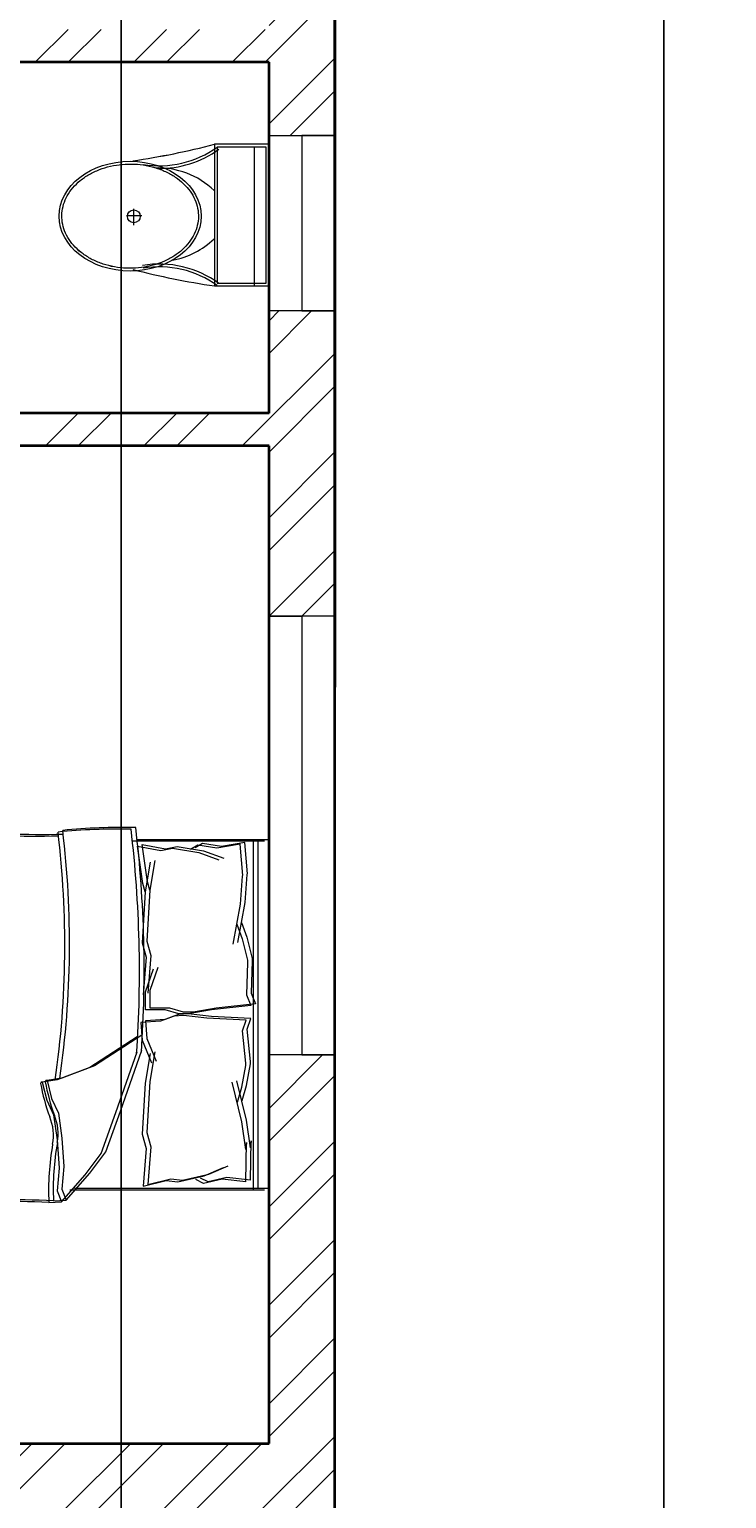
# Model space of a CAD drawing. Units: inches. Extents: x 2120 to 4013, y 1390 to 3019.
# Tile 43 of 59: x 2968 to 3063, y 1964 to 2165. Entities that reach past the tile are written whole.
import ezdxf

# ---------------------------------------------------------------- set-up
doc = ezdxf.new("R2010")
doc.units = ezdxf.units.IN
for name, color, linetype, lineweight in [('A-ANNO-DIMS', 2, 'Continuous', 18), ('A-FLOR-FIXT', 9, 'Continuous', 18), ('A-FURN', 8, 'Continuous', 13), ('A-GLAZ', 4, 'Continuous', 18), ('A-WALL', 7, 'Continuous', 35), ('A-WALL-PATT', 252, 'Continuous', 13)]:
    doc.layers.add(name, color=color, linetype=linetype, lineweight=lineweight)
doc.styles.get("Standard").update_dxf_attribs({"font": 'arial.ttf'})
doc.dimstyles.get("Standard").update_dxf_attribs({"dimtxt": 0.18, "dimasz": 0.18, "dimexe": 0.18, "dimexo": 0.0625, "dimgap": 0.09, "dimtad": 0, "dimtih": 1, "dimtoh": 1, "dimdec": 4, "dimzin": 0, "dimdsep": 46, "dimtxsty": 'Standard', "dimcen": 0.09, "dimadec": 0, "dimazin": 0, "dimtfac": 1, "dimtdec": 4, "dimtofl": 0, "dimtmove": 0, "dimatfit": 3, "dimfxl": 1, "dimtolj": 1, "dimtzin": 0, "dimarcsym": 0})

# ---------------------------------------------------------------- blocks, each defined once
blk = doc.blocks.new('A$C31115884')
for p, q in [((283.1, 497.7), (223.4, 497.7)), ((257.5, 466.4), (257.5, 523.2)), ((0, 200), (0, 0)), ((520, 200), (0, 200)), ((10, 190), (10, 10)), ((510, 190), (10, 190)), ((510, 10), (510, 190)), ((520, 0), (520, 200)), ((510, 54.5), (0, 54.5)), ((10, 10), (510, 10)), ((0, 0), (520, 0))]:
    blk.add_line(p, q)
blk.add_circle((255.6, 496.4), 23.6)
for centre, radius, start, end in [((2777.7, -204.6), 2807, 165.4549, 171.7133), ((3237, 905), 2807, 188.2867, 194.5451), ((-294.5, 403.3), 364.7, 324.2091, 9.3499), ((-294.5, 403.3), 374.7, 324.2091, 9.3499), ((805.8, 403.3), 364.7, 170.6501, 215.7909), ((139.5, 406.2), 293.5, 315.8436, 2.6563), ((805.8, 403.3), 374.7, 179.2036, 215.7909), ((383.6, 406.2), 293.5, 190.2774, 224.1564)]:
    blk.add_arc(centre, radius, start, end)
blk.add_ellipse((256.2, 509.9), major_axis=(0, -260.7), ratio=0.772727)
blk.add_open_spline([(256.2, 259.2), (263.1, 259.2), (270, 259.7), (287.8, 262.3), (298.7, 265.1), (319.9, 273.1), (330.2, 278.4), (350.1, 291.1), (359.7, 298.7), (377.7, 315.9), (386.2, 325.5), (401.7, 346.6), (408.8, 358.1), (421.3, 382.5), (426.8, 395.5), (435.9, 422.4), (439.5, 436.4), (444.8, 465.1), (446.5, 479.7), (447.9, 509.2), (447.6, 524), (445, 553.3), (442.7, 567.8), (436.3, 596), (432.1, 609.7), (421.9, 636), (416, 648.6), (402.5, 672.1), (395, 683), (378.6, 703), (369.8, 712.1), (351.1, 728), (341.3, 734.8), (320.9, 746.2), (310.4, 750.7), (288.9, 757.3), (278, 759.4), (256, 761), (245, 760.6), (223.1, 757.2), (212.3, 754.3), (191.1, 746.1), (180.8, 740.7), (160.9, 727.8), (151.4, 720.1), (133.5, 702.7), (125.1, 693), (109.6, 671.7), (102.6, 660.2), (90.2, 635.7), (84.9, 622.7), (76, 595.6), (72.4, 581.6), (67.2, 552.9), (65.6, 538.2), (64.4, 508.8), (64.8, 494), (67.5, 464.7), (69.9, 450.2), (76.6, 422), (80.8, 408.3), (91.1, 382.2), (97.2, 369.7), (110.8, 346.3), (118.4, 335.4), (134.8, 315.6), (143.7, 306.7), (162.4, 290.9), (172.3, 284.2), (192.8, 273), (203.3, 268.6), (224.8, 262.2), (235.8, 260.2), (249.9, 259.3), (253, 259.2), (256.2, 259.2)], degree=3, knots=[0, 0, 0, 0, 0.110105, 0.110105, 0.285049, 0.285049, 0.459994, 0.459994, 0.634938, 0.634938, 0.809882, 0.809882, 0.984827, 0.984827, 1.159771, 1.159771, 1.334715, 1.334715, 1.50966, 1.50966, 1.684604, 1.684604, 1.859549, 1.859549, 2.034493, 2.034493, 2.209437, 2.209437, 2.384382, 2.384382, 2.559326, 2.559326, 2.73427, 2.73427, 2.909215, 2.909215, 3.084159, 3.084159, 3.259103, 3.259103, 3.434048, 3.434048, 3.608992, 3.608992, 3.783936, 3.783936, 3.958881, 3.958881, 4.133825, 4.133825, 4.30877, 4.30877, 4.483714, 4.483714, 4.658658, 4.658658, 4.833603, 4.833603, 5.008547, 5.008547, 5.183491, 5.183491, 5.358436, 5.358436, 5.53338, 5.53338, 5.708324, 5.708324, 5.883269, 5.883269, 6.058213, 6.058213, 6.233158, 6.233158, 6.283185, 6.283185, 6.283185, 6.283185])
blk = doc.blocks.new('BED-DOUBLE-PLAN')
for p, q in [((3.48, 63.34), (3.48, 81.45)), ((3.48, 81.45), (51.27, 81.45)), ((3.7, 62.7), (3.7, 80.81)), ((51.27, 81.45), (51.27, 54.84)), ((51.5, 80.81), (51.5, 54.2)), ((3.48, 79.91), (51.27, 79.91)), ((3.7, 79.27), (51.5, 79.27)), ((3.9, 78.11), (8.18, 78.44)), ((8.18, 78.44), (8.29, 78.42)), ((8.29, 78.42), (12.11, 78.13)), ((14.86, 77.7), (16.88, 78.42)), ((16.88, 78.42), (19.77, 79.14)), ((17.11, 77.78), (20, 78.5)), ((19.77, 79.14), (20.09, 79.14)), ((20, 78.5), (20.32, 78.5)), ((20.09, 79.14), (24.54, 79)), ((20.32, 78.5), (24.77, 78.36)), ((24.54, 79), (25.98, 79.58)), ((24.77, 78.36), (26.21, 78.94)), ((25.98, 79.58), (26.56, 74.23)), ((26.21, 78.94), (26.79, 73.59)), ((27.98, 78.95), (27.73, 73.58)), ((29.46, 78.47), (27.98, 78.95)), ((33.89, 78.89), (29.46, 78.47)), ((34.21, 78.91), (33.89, 78.89)), ((37.14, 78.37), (34.21, 78.91)), ((45.71, 78.9), (41.92, 78.38)), ((50.11, 78.89), (44.71, 78.99)), ((44.71, 78.99), (45.71, 78.9)), ((50.11, 78.89), (49.73, 75.68)), ((3.9, 78.13), (4.47, 74.95)), ((4.12, 77.49), (4.7, 74.31)), ((4.13, 77.47), (8.41, 77.8)), ((8.41, 77.8), (8.51, 77.78)), ((8.51, 77.78), (12.34, 77.49)), ((12.11, 78.13), (17.6, 77.12)), ((12.34, 77.49), (17.83, 76.48)), ((15.08, 77.06), (17.11, 77.78)), ((28.21, 78.32), (27.96, 72.94)), ((29.69, 77.83), (28.21, 78.32)), ((34.11, 78.25), (29.69, 77.83)), ((34.43, 78.27), (34.11, 78.25)), ((37.37, 77.73), (34.43, 78.27)), ((41.92, 78.38), (36.5, 77.02)), ((42.14, 77.74), (36.72, 76.38)), ((39.2, 77.77), (37.14, 78.37)), ((39.43, 77.13), (37.37, 77.73)), ((45.94, 78.26), (42.14, 77.74)), ((50.34, 78.25), (44.94, 78.35)), ((44.94, 78.35), (45.94, 78.26)), ((50.34, 78.25), (49.96, 75.04)), ((4.47, 74.95), (4.04, 72.35)), ((5.05, 72.49), (6.06, 75.24)), ((5.28, 71.85), (6.29, 74.6)), ((49.31, 73.19), (48.13, 75.87)), ((49.54, 72.55), (48.36, 75.23)), ((49.73, 75.68), (50.33, 73.11)), ((49.96, 75.04), (50.56, 72.47)), ((4.7, 74.31), (4.27, 71.71)), ((4.47, 68.88), (5.05, 72.49)), ((26.56, 74.23), (27.14, 71.05)), ((26.79, 73.59), (27.37, 70.41)), ((27.73, 73.58), (27.36, 70.37)), ((27.96, 72.94), (27.58, 69.73)), ((50.11, 69.62), (49.31, 73.19)), ((50.34, 68.98), (49.54, 72.55)), ((50.33, 73.11), (49.82, 72.06)), ((50.56, 72.47), (50.04, 71.42)), ((4.04, 72.35), (4.62, 71.33)), ((4.27, 71.71), (4.85, 70.7)), ((4.7, 68.24), (5.28, 71.85)), ((27.14, 71.05), (27.14, 69.74)), ((27.36, 70.37), (27.44, 69.07)), ((27.37, 70.41), (27.37, 69.1)), ((4.76, 67.29), (4.47, 68.88)), ((27.14, 69.74), (26.56, 67.86)), ((27.37, 69.1), (26.79, 67.23)), ((27.44, 69.07), (28.13, 67.23)), ((27.58, 69.73), (27.67, 68.43)), ((27.67, 68.43), (28.36, 66.59)), ((49.92, 68.01), (50.11, 69.62)), ((50.15, 67.37), (50.34, 68.98)), ((4.19, 64.11), (4.76, 67.29)), ((4.41, 63.47), (4.99, 66.65)), ((4.99, 66.65), (4.7, 68.24)), ((26.56, 67.86), (26.56, 65.18)), ((26.79, 67.23), (26.79, 64.54)), ((28.13, 67.23), (28.3, 64.55)), ((28.36, 66.59), (28.53, 63.91)), ((50.7, 64.87), (49.92, 68.01)), ((50.93, 64.23), (50.15, 67.37)), ((9.28, 64.83), (4.19, 64.11)), ((6.38, 65.82), (10.42, 65.15)), ((6.61, 65.18), (10.64, 64.51)), ((10.42, 65.15), (9.28, 64.83)), ((10.64, 64.51), (9.51, 64.19)), ((10.42, 65.15), (17.43, 64.72)), ((10.64, 64.51), (17.65, 64.08)), ((17.43, 64.72), (19.39, 65.28)), ((17.65, 64.08), (19.61, 64.64)), ((19.39, 65.28), (24.52, 64.87)), ((19.61, 64.64), (24.75, 64.23)), ((24.1, 65.18), (20.96, 66.27)), ((24.33, 64.54), (21.19, 65.63)), ((26.56, 65.18), (24.1, 65.18)), ((26.79, 64.54), (24.33, 64.54)), ((28.3, 64.55), (30.75, 64.71)), ((30.75, 64.71), (33.82, 65.99)), ((30.98, 64.07), (34.05, 65.35)), ((32.57, 65.82), (36.6, 65.15)), ((32.79, 65.18), (36.83, 64.51)), ((36.6, 65.15), (43.61, 64.72)), ((36.83, 64.51), (43.84, 64.08)), ((43.61, 64.72), (45.57, 65.28)), ((43.84, 64.08), (45.8, 64.64)), ((45.57, 65.28), (50.7, 64.87)), ((45.8, 64.64), (50.93, 64.23)), ((9.51, 64.19), (4.41, 63.47)), ((28.53, 63.91), (30.98, 64.07)), ((30.26, 64.06), (34.45, 57.57)), ((30.49, 63.42), (34.68, 56.93)), ((40.65, 61.13), (32.31, 64.06)), ((40.87, 60.49), (32.54, 63.42)), ((46.22, 59.12), (40.65, 61.13)), ((46.45, 58.48), (40.87, 60.49)), ((49.16, 56.95), (46.22, 59.12)), ((49.39, 56.31), (46.45, 58.48)), ((34.45, 57.57), (36.15, 53.08)), ((34.68, 56.93), (36.38, 52.44)), ((52.87, 53.7), (49.16, 56.95)), ((53.1, 53.06), (49.39, 56.31)), ((36.15, 53.08), (36.46, 51.07)), ((36.38, 52.44), (36.69, 50.43)), ((38.94, 51.69), (40.96, 52.62)), ((40.96, 52.62), (44.36, 53.08)), ((41.18, 51.98), (44.59, 52.44)), ((44.36, 53.08), (48.23, 53.39)), ((44.59, 52.44), (48.46, 52.75)), ((48.23, 53.39), (51.33, 53.08)), ((48.46, 52.75), (51.56, 52.44)), ((51.33, 53.08), (52.87, 53.7)), ((51.56, 52.44), (53.1, 53.06)), ((52.95, 51.96), (52.87, 53.7, 3.87)), ((53.18, 51.32), (53.1, 53.06, 3.87)), ((36.46, 51.07), (38.94, 51.69)), ((36.69, 50.43), (39.17, 51.05)), ((39.17, 51.05), (41.18, 51.98)), ((15.06, 2.2), (39.68, 2.2)), ((15.29, 1.56), (39.91, 1.56))]:
    blk.add_line(p, q)
for centre, radius, start, end in [((21.36, -100.61), 164.97, 86.0865, 96.7821), ((85.16, 61.35), 83.31, 178.7218, 185.604), ((85.39, 60.71), 83.31, 178.7218, 185.604), ((21.59, -101.25), 164.97, 86.0865, 96.7821), ((17.76, -74.87), 129.02, 81.7845, 96.9006), ((17.99, -75.51), 129.02, 81.7845, 96.9006), ((-167.31, 50.27), 170.11, 358.4762, 1.0082), ((-167.08, 49.63), 170.11, 358.4762, 1.0082), ((43.74, 46.38), 6.22, 78.6608, 113.7384), ((51.33, 88.1), 36.18, 259.8763, 272.5657), ((36.64, 51.01), 0.185, 160.2464, 271.1377), ((31.16, 79.96), 29.65, 280.6617, 289.8806), ((36.87, 50.37), 0.185, 160.2464, 271.1377), ((31.38, 79.32), 29.65, 280.6617, 289.8806), ((43.97, 45.74), 6.22, 78.6608, 113.7384), ((51.56, 87.46), 36.18, 259.8763, 272.5657), ((182.27, 45.13), 129.5, 176.9791, 183.8365), ((182.5, 44.49), 129.5, 176.9791, 183.8365), ((484.82, 30.83), 482.31, 178.2277, 181.7185), ((485.05, 30.19), 482.31, 178.2277, 181.7185), ((-4508.74, 13.62), 4561.86, 0.00217, 0.28689), ((-4508.51, 12.99), 4561.86, 0.00217, 0.28689), ((-26.9, 16.93), 29.63, 346.0648, 358.9113), ((-26.67, 16.29), 29.63, 346.0648, 358.9113), ((76.16, 12.78), 23.07, 177.4714, 206.4681), ((76.39, 12.14), 23.07, 177.4714, 206.4681), ((-21.66, 11.17), 23.56, 337.9751, 356.652), ((-21.43, 10.53), 23.56, 337.9751, 356.652), ((1.09, 1.73), 1.09, 146.1736, 293.4781), ((21.43, -119.39), 121.76, 92.9958, 99.4091), ((-17.22, 105.16), 106.46, 283.3832, 287.7053), ((-16.99, 104.52), 106.46, 283.3832, 287.7053), ((41.15, -130.83), 133.04, 84.4998, 90.6351), ((54.41, 2.58), 1.1, 242.6588, 356.02), ((1.32, 1.09), 1.09, 146.1736, 293.4781), ((21.66, -120.03), 121.76, 92.9958, 99.4091), ((41.38, -131.47), 133.04, 84.4998, 90.6351), ((54.64, 1.94), 1.1, 242.6588, 356.02)]:
    blk.add_arc(centre, radius, start, end)
blk = doc.blocks.new('WIN-PLAN-24IN-02')
for p, q in [((0, 0), (0, 9)), ((0, 9), (0, 4.5)), ((24, 4.5), (24, 9)), ((24, 9), (24, 0)), ((0, 4.5), (24, 4.5))]:
    blk.add_line(p, q)
blk = doc.blocks.new('WIN-PLAN-60IN')
for p, q in [((0, 9), (0, 0)), ((60, 4.5), (60, 9)), ((60, 9), (60, 0)), ((0, 0), (0, 4.5)), ((0, 4.5), (60, 4.5))]:
    blk.add_line(p, q)
blk = doc.blocks.new('*D212')
at = {"layer": 'A-ANNO-DIMS', "color": 0, "lineweight": -2, "transparency": 16777216}
for p, q in [((3009.8, 2352.53), (3054.91, 2352.53)), ((3054.73, 2352.35), (3054.73, 1947.71)), ((3054.73, 1542.71), (3054.73, 1947.35)), ((3009.8, 1542.53), (3054.91, 1542.53))]:
    blk.add_line(p, q, dxfattribs=at)
at = {"layer": 'A-ANNO-DIMS', "color": 0, "transparency": 16777216}
for points in [[(3054.7, 2352.35), (3054.76, 2352.35), (3054.73, 2352.53)], [(3054.7, 1542.71), (3054.76, 1542.71), (3054.73, 1542.53)]]:
    blk.add_solid(points, dxfattribs=at)
at = {"layer": 'Defpoints', "color": 0, "transparency": 16777216}
for p in [(3009.73, 2352.53), (3009.73, 1542.53), (3054.73, 1542.53)]:
    blk.add_point(p, dxfattribs=at)
at = {"layer": 'A-ANNO-DIMS', "color": 0, "transparency": 16777216, "insert": (3054.73, 1947.53), "char_height": 0.18, "attachment_point": 5}
blk.add_mtext('\\A1;810', dxfattribs=at)
blk = doc.blocks.new('*D217')
at = {"layer": 'A-ANNO-DIMS', "color": 0, "lineweight": -2, "transparency": 16777216}
for p, q in [((3071.67, 2352.53), (2980.31, 2352.53)), ((2980.49, 2352.35), (2980.49, 1947.71)), ((2980.49, 1542.71), (2980.49, 1947.35)), ((3305.67, 1542.53), (2980.31, 1542.53))]:
    blk.add_line(p, q, dxfattribs=at)
at = {"layer": 'A-ANNO-DIMS', "color": 0, "transparency": 16777216}
for points in [[(2980.46, 2352.35), (2980.52, 2352.35), (2980.49, 2352.53)], [(2980.46, 1542.71), (2980.52, 1542.71), (2980.49, 1542.53)]]:
    blk.add_solid(points, dxfattribs=at)
at = {"layer": 'Defpoints', "color": 0, "transparency": 16777216}
for p in [(2980.49, 2352.53), (3071.73, 2352.53), (3305.73, 1542.53)]:
    blk.add_point(p, dxfattribs=at)
at = {"layer": 'A-ANNO-DIMS', "color": 0, "transparency": 16777216, "insert": (2980.49, 1947.53), "char_height": 0.18, "attachment_point": 5}
blk.add_mtext('\\A1;810', dxfattribs=at)

msp = doc.modelspace()

# ---------------------------------------------------------------- hatches: boundary and pattern name
at = {"layer": 'A-WALL-PATT'}
h = msp.add_hatch(dxfattribs=at)
h.set_pattern_fill('ANSI32', color=256)
h.paths.add_polyline_path([(2271.7331, 2122.6377), (2262.7331, 2122.6377), (2262.7331, 2040.3893), (2267.2331, 2040.3893), (2271.7331, 2040.3893), (2271.7331, 2044.8856), (2271.7331, 2070.531), (2391.7331, 2070.531), (2391.7331, 1926.5306), (2388.3993, 1926.5306), (2388.3993, 1922.531), (2395.7331, 1922.531), (2395.7331, 1992.531), (2400.4511, 1992.531), (2400.4511, 1997.0306), (2395.7331, 1997.0306), (2395.7331, 2070.531), (2443.7331, 2070.531), (2443.7331, 2046.1368), (2448.2331, 2046.1368), (2448.2331, 2070.531), (2580.2331, 2070.531), (2580.2331, 1997.0306), (2492.9076, 1997.0306), (2492.9076, 1992.531), (2580.2331, 1992.531), (2580.2331, 1983.9368), (2589.2331, 1983.9368), (2589.2331, 2070.531), (2589.2331, 2075.0306), (2396.2331, 2075.0306), (2396.2331, 2184.3565), (2393.9831, 2184.3565), (2391.7331, 2184.3565), (2391.7331, 2075.0306), (2271.7331, 2075.0306)])
h.paths.add_polyline_path([(2724.7331, 2138.0306), (2628.7331, 2138.0306), (2628.7331, 2070.5306), (2628.7331, 2067.0987), (2633.2331, 2067.0987), (2637.7331, 2067.0987), (2637.7331, 2070.531), (2657.3413, 2070.531), (2657.3413, 2079.5306), (2637.7331, 2079.5306), (2637.7331, 2129.031), (2715.7331, 2129.031), (2715.7331, 2079.5306), (2698.0378, 2079.5306), (2698.0378, 2070.531), (2715.7331, 2070.531), (2715.7331, 2012.1531), (2720.2331, 2012.1531), (2724.7331, 2012.1531)])
h.paths.add_polyline_path([(2724.7331, 2213.031), (2831.3209, 2213.031), (2831.3209, 2215.281), (2831.3209, 2217.5306), (2724.7331, 2217.5306), (2724.7331, 2343.531), (2751.8755, 2343.531), (2751.8755, 2352.5306), (2715.7331, 2352.5306), (2715.7331, 2138.031), (2724.7331, 2138.031)])
h.paths.add_polyline_path([(2902.53, 2352.5306), (2811.8755, 2352.5306), (2811.8755, 2343.531), (2867.2331, 2343.531), (2867.2331, 2217.5306), (2863.6364, 2217.5306), (2863.6364, 2213.031), (2871.7331, 2213.031), (2871.7331, 2217.531), (2871.7331, 2343.531), (2902.53, 2343.531)])
h.paths.add_polyline_path([(3009.7331, 2352.5306), (2938.53, 2352.5306), (2938.53, 2343.531), (2966.2331, 2343.531), (2966.2331, 2242.3281), (2968.4831, 2242.3281), (2970.7331, 2242.3281), (2970.7331, 2343.531), (3009.7331, 2343.531)])
h.paths.add_polyline_path([(3009.7331, 2217.5306), (2970.7331, 2217.5306), (2970.7331, 2220.5422), (2968.4831, 2220.5422), (2966.2331, 2220.5422), (2966.2331, 2217.5306), (2911.7752, 2217.5306), (2907.7331, 2217.5306), (2907.7331, 2213.0306), (2907.7331, 2194.9663), (2912.2331, 2194.9663), (2912.2331, 2213.031), (2970.7331, 2213.031), (3000.7331, 2213.031), (3000.7331, 2205.523), (3009.7331, 2205.523)])
h.paths.add_polyline_path([(3009.7331, 2181.5227), (3000.7331, 2181.5227), (3000.7331, 2165.0306), (2912.2331, 2165.0306), (2912.2331, 2170.8202), (2907.7331, 2170.8202), (2907.7331, 2165.0306), (2899.5169, 2165.0306), (2899.5169, 2162.7806), (2899.5169, 2160.531), (2907.7331, 2160.531), (2907.7331, 2137.3432), (2912.2331, 2137.3432), (2912.2331, 2160.531), (3000.7331, 2160.531), (3000.7331, 2150.4993), (3009.7331, 2150.4993)])
h.paths.add_polyline_path([(3009.7331, 2126.499), (3005.2331, 2126.499), (3000.7331, 2126.499), (3000.7331, 2112.5306), (2912.2331, 2112.5306), (2912.2331, 2115.6036), (2907.7331, 2115.6036), (2907.7331, 2108.031), (3000.7331, 2108.031), (3000.7331, 2084.7256), (3009.7331, 2084.7256)], flags=17)
h.paths.add_polyline_path([(3009.7331, 1971.531), (3009.7331, 2024.7253), (3000.7331, 2024.7253), (3000.7331, 2006.4153), (3000.7331, 1971.5306), (2864.2331, 1971.5306), (2864.2331, 2160.531), (2868.0522, 2160.531), (2868.0522, 2165.0306), (2859.7331, 2165.0306), (2859.7331, 1971.5306), (2724.7331, 1971.5306), (2724.7331, 1977.7012), (2715.7331, 1977.7012), (2715.7331, 1962.5306), (2715.7331, 1950.9035), (2720.2331, 1950.9035), (2724.7331, 1950.9035), (2724.7331, 1962.531), (2855.2331, 1962.531), (2859.7331, 1962.531), (2859.7331, 1835.031), (2864.2331, 1834.8158), (2864.2331, 1962.531), (2958.7331, 1962.531), (2958.7331, 1937.0925), (2963.2331, 1937.0925), (2963.2331, 1962.531), (3000.7331, 1962.531), (3009.7331, 1962.531)])
h.paths.add_polyline_path([(2724.7331, 1728.531), (2822.7164, 1728.531), (2822.7164, 1733.0306), (2724.7331, 1733.0306), (2724.7331, 1779.3416), (2715.7331, 1779.3416), (2715.7331, 1581.531), (2753.02, 1581.531), (2753.02, 1586.031), (2753.02, 1590.5306), (2724.7331, 1590.5306)])
h.paths.add_polyline_path([(2864.2331, 1590.531), (2864.2331, 1787.031), (2868.4075, 1787.031), (2868.4075, 1791.5306), (2859.7331, 1791.5306), (2859.7331, 1739.0306), (2859.7331, 1733.0306), (2854.3125, 1733.0306), (2854.3125, 1728.531), (2859.7331, 1728.531), (2859.7331, 1590.5306), (2813.02, 1590.5306), (2813.02, 1581.531), (2868.4123, 1581.531), (2868.4123, 1583.781), (2868.4123, 1586.0306), (2864.2331, 1586.0306)])
h.paths.add_polyline_path([(3009.7331, 1754.6619), (3000.7331, 1754.6619), (3000.7331, 1739.0306), (2912.2331, 1739.0306), (2912.2331, 1742.2257), (2907.7331, 1742.2257), (2907.7331, 1739.0306), (2907.7331, 1734.531), (3000.7331, 1734.531), (3000.7331, 1590.5306), (3000.7331, 1586.0306), (2971.3921, 1586.0306), (2971.3921, 1581.531), (3009.7331, 1581.531)])
h.paths.add_polyline_path([(2911.3921, 1583.781), (2911.3921, 1586.0306), (2891.2138, 1586.0306), (2891.2138, 1581.531), (2911.3921, 1581.531)])
h.paths.add_polyline_path([(3009.7331, 1799.8422), (3000.7331, 1799.8422), (3000.7331, 1791.5306), (2912.2331, 1791.5306), (2912.2331, 1796.3264), (2909.9831, 1796.3264), (2907.7331, 1796.3264), (2907.7331, 1791.5306), (2902.7033, 1791.5306), (2902.7033, 1787.031), (2907.7331, 1787.031), (2907.7331, 1761.1622), (2912.2331, 1761.1622), (2912.2331, 1787.031), (3000.7331, 1787.031), (3000.7331, 1778.6622), (3009.7331, 1778.6622)])
h.paths.add_polyline_path([(3009.7331, 1839.5306), (2963.2331, 1839.5306), (2963.2331, 1842.8629), (2960.9831, 1842.8629), (2958.7331, 1842.8629), (2958.7331, 1839.5306), (2907.7331, 1839.5306), (2907.7331, 1814.4599), (2912.2331, 1814.4599), (2912.2331, 1835.031), (3000.7331, 1835.031), (3000.7331, 1823.8425), (3009.7331, 1823.8425), (3009.7331, 1835.031)])
h.paths.add_polyline_path([(2963.2331, 1901.0922), (2960.9831, 1901.0922), (2958.7331, 1901.0922), (2958.7331, 1862.8843), (2963.2331, 1862.8843)], flags=17)
h.paths.add_polyline_path([(2724.7331, 1891.9826), (2724.7331, 1914.3416), (2715.7331, 1914.3416), (2715.7331, 1783.8416), (2637.7331, 1783.8416), (2637.7331, 1914.3416), (2628.7331, 1914.3416), (2624.7701, 1914.3416), (2624.7701, 1909.8416), (2624.7701, 1905.3419), (2628.7331, 1905.3419), (2628.7331, 1876.9915), (2628.7331, 1779.3419), (2637.7331, 1779.3419), (2715.7331, 1779.3419), (2724.7331, 1779.3419), (2724.7331, 1835.031)])
h.paths.add_polyline_path([(2637.7331, 1731.531), (2637.7331, 1779.3416), (2628.7331, 1779.3416), (2628.7331, 1731.5306), (2589.2331, 1731.5306), (2535.9814, 1731.5306), (2496.7331, 1731.5306), (2496.7331, 1725.6876), (2498.9831, 1725.6876), (2501.2331, 1725.6876), (2501.2331, 1727.031), (2628.7331, 1727.031), (2628.7331, 1680.4203), (2628.7331, 1590.5306), (2628.7331, 1586.0306), (2604.1361, 1586.0306), (2604.1361, 1581.531), (2637.7331, 1581.531), (2637.7331, 1590.531)])

# ---------------------------------------------------------------- linework, layer by layer
at = {"layer": 'A-WALL'}
for p, q in [((3009.7331, 2352.531), (3009.7331, 2075.031)), ((3009.7331, 2352.5306), (3009.7331, 2075.0306)), ((3009.7331, 1971.531), (3009.7331, 2182.408)), ((3009.7331, 1971.5306), (3009.7331, 2182.4077)), ((3000.7331, 2160.531), (2912.2331, 2160.531)), ((3000.7331, 2160.5306), (2912.2331, 2160.5306)), ((3000.7331, 2112.531), (3000.7331, 2160.531)), ((3000.7331, 2112.5306), (3000.7331, 2160.5306)), ((3000.7331, 2112.531), (2912.2331, 2112.531)), ((3000.7331, 2112.5306), (2912.2331, 2112.5306)), ((3000.7331, 2108.031), (2907.7331, 2108.031)), ((3000.7331, 2108.0306), (2907.7331, 2108.0306)), ((3000.7331, 1971.531), (3000.7331, 2108.031)), ((3000.7331, 1971.5306), (3000.7331, 2108.0306)), ((2864.2331, 1971.531), (3000.7331, 1971.531)), ((2864.2331, 1971.5306), (3000.7331, 1971.5306)), ((3009.7331, 1962.531), (3009.7331, 1971.531)), ((3009.7331, 1962.5306), (3009.7331, 1971.5306))]:
    msp.add_line(p, q, dxfattribs=at)

# ---------------------------------------------------------------- block references
at = {"layer": 'A-FLOR-FIXT', "xscale": 0.0372717239612423, "yscale": 0.0372717239612423, "zscale": 0.0372717239612423, "rotation": 89.99999999999999}
for p in [(3000.7331, 2129.9279), (3000.7331, 2129.9276)]:
    msp.add_blockref('A$C31115884', p, dxfattribs=at)
at = {"layer": 'A-FURN'}
for p, rotation in [((2919.2869, 2057.6824), 270.0000000000001), ((2919.2869, 2057.6821), 270)]:
    msp.add_blockref('BED-DOUBLE-PLAN', p, dxfattribs=dict(at, rotation=rotation))
at = {"layer": 'A-GLAZ'}
for name, p, rotation in [('WIN-PLAN-24IN-02', (3000.7331, 2150.4993), 270), ('WIN-PLAN-24IN-02', (3000.7331, 2150.499), 269.9999999999973), ('WIN-PLAN-60IN', (3000.7331, 2084.7256), 270), ('WIN-PLAN-60IN', (3000.7331, 2084.7253), 269.9999999999983)]:
    msp.add_blockref(name, p, dxfattribs=dict(at, rotation=rotation))

# ---------------------------------------------------------------- dimensions: what is measured, and where the dimension line sits
at = {"layer": 'A-ANNO-DIMS'}
for base, p1, p2, picture, middle in [((2980.4877, 2352.531), (3305.7347, 1542.531), (3071.7347, 2352.531), '*D217', (2980.4877, 1947.531)), ((3054.7331, 1542.531), (3009.7331, 2352.531), (3009.7331, 1542.531), '*D212', (3054.7331, 1947.531))]:
    dim = msp.add_linear_dim(base=base, p1=p1, p2=p2, angle=90, dimstyle='Standard', override={"dimdec": 0, "dimlfac": 1, "dimrnd": 0, "dimzin": 0, "dimdsep": 46, "dimlunit": 2}, dxfattribs=at)
    dim.commit()
    dim.dimension.update_dxf_attribs({"geometry": picture, "text_midpoint": middle})

doc.saveas('drawing.dxf')
